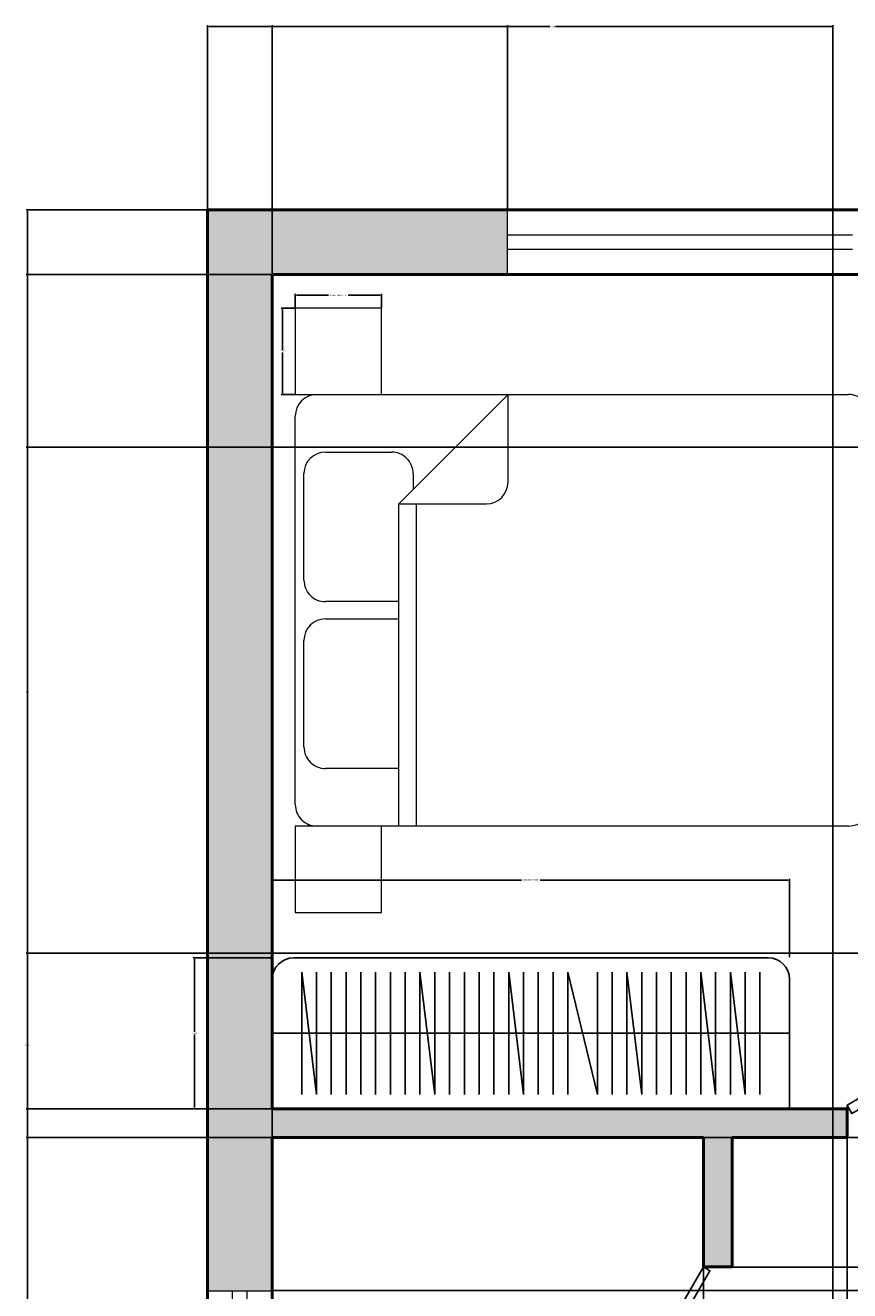
# Model space of a CAD drawing. Units: inches. Extents: x 3439 to 3988, y 1915 to 2284.
# Tile 2 of 7: x 3439 to 3554, y 2108 to 2284. Entities that reach past the tile are written whole.
import ezdxf

# ---------------------------------------------------------------- set-up
doc = ezdxf.new("R2010")
doc.units = ezdxf.units.IN
for name, color, linetype, lineweight in [('A-ANNO-DIMS', 2, 'Continuous', 18), ('A-DOOR', 3, 'Continuous', 25), ('A-FLOR-CASE', 8, 'Continuous', 25), ('A-FURN', 9, 'Continuous', 18), ('A-GLAZ', 4, 'Continuous', 18), ('A-WALL', 7, 'Continuous', 50)]:
    doc.layers.add(name, color=color, linetype=linetype, lineweight=lineweight)
doc.layers.add('A-WALL-PATT', color=18, linetype='Continuous', lineweight=13, true_color=0x000000)
doc.styles.get("Standard").update_dxf_attribs({"font": 'arial.ttf'})
doc.dimstyles.get("Standard").update_dxf_attribs({"dimtxt": 0.18, "dimasz": 0.18, "dimexe": 0.18, "dimexo": 0.0625, "dimgap": 0.09, "dimtad": 0, "dimtih": 1, "dimtoh": 1, "dimdec": 4, "dimzin": 0, "dimdsep": 46, "dimtxsty": 'Standard', "dimcen": 0.09, "dimadec": 0, "dimazin": 0, "dimtfac": 1, "dimtdec": 4, "dimtofl": 0, "dimtmove": 0, "dimatfit": 3, "dimfxl": 1, "dimtolj": 1, "dimtzin": 0, "dimarcsym": 0})

# ---------------------------------------------------------------- blocks, each defined once
blk = doc.blocks.new('*U4')
for p, q in [((0, 0), (0, -6)), ((40, 0), (40, -6))]:
    blk.add_line(p, q)
blk.add_lwpolyline([(0, 0), (34.64, 20), (35.52, 18.48), (0.87, -1.52)], close=True)
blk.add_arc((0, 0), 40, 0, 30)
blk = doc.blocks.new('*U5')
for p, q in [((0, 0), (0, 6)), ((40, 0), (40, 6))]:
    blk.add_line(p, q)
blk.add_lwpolyline([(0, 0), (34.64, -20), (35.52, -18.48), (0.87, 1.52)], close=True)
blk.add_arc((0, 0), 40, 330, 0)
blk = doc.blocks.new('Bed - Queen')
for p, q in [((3, 0), (56.99999, 0)), ((10.99999, -1.2), (25.79998, -1.2)), ((34.19999, -1.2), (48.99999, -1.2)), ((0, -77.00003), (0, -3)), ((59.99999, -3), (59.99999, -77.00003)), ((7.99999, -14.4), (7.99999, -4.2)), ((28.79998, -4.2), (28.79998, -14.4)), ((31.19999, -14.4), (31.19999, -4.2)), ((51.99999, -4.2), (51.99999, -13.4)), ((0, -14.4), (44.8, -14.4)), ((59.99999, -29.6), (44.8, -14.4)), ((44.8, -14.4), (44.8, -26.6)), ((44.8, -16.8), (0, -16.8)), ((48.99999, -16.4), (46.79936, -16.4)), ((47.8, -29.6), (59.99999, -29.6)), ((56.99999, -80.00003), (3, -80.00003))]:
    blk.add_line(p, q)
for centre, start, end in [((3, -3), 90, 180), ((56.99999, -3), 0, 90), ((10.99999, -4.2), 90, 180), ((25.79998, -4.2), 0, 90), ((34.19999, -4.2), 90, 180), ((48.99999, -4.2), 0, 90), ((48.99999, -13.4), 270, 0), ((47.8, -26.6), 180, 270), ((3, -77.00003), 180, 270), ((56.99999, -77.00003), 270, 0)]:
    blk.add_arc(centre, 3, start, end)
blk = doc.blocks.new('WINDOW-GLASS-48IN')
for p, q in [((0, 2), (48, 2)), ((0, 0), (48, 0))]:
    blk.add_line(p, q)
blk = doc.blocks.new('WINDOW-GLASS-24IN')
for p, q in [((0, 2), (24, 2)), ((0, 0), (24, 0))]:
    blk.add_line(p, q)
blk = doc.blocks.new('WARDROBE-72IN')
for p, q in [((3, 21), (69, 21)), ((0, 0), (0, 18)), ((4.11, 2), (4.11, 19)), ((4.11, 19), (6.17, 2)), ((6.17, 2), (6.17, 19)), ((8.23, 2), (8.23, 19)), ((10.28, 2), (10.28, 19)), ((12.34, 2), (12.34, 19)), ((14.4, 2), (14.4, 19)), ((16.45, 2), (16.45, 19)), ((18.51, 2), (18.51, 19)), ((20.57, 2), (20.57, 19)), ((20.57, 19), (22.62, 2)), ((22.62, 2), (22.62, 19)), ((24.68, 2), (24.68, 19)), ((26.74, 2), (26.74, 19)), ((28.79, 2), (28.79, 19)), ((30.85, 2), (30.85, 19)), ((32.91, 2), (32.91, 19)), ((32.91, 19), (34.97, 2)), ((34.97, 2), (34.97, 19)), ((37.02, 2), (37.02, 19)), ((39.08, 2), (39.08, 19)), ((41.14, 2), (41.14, 19)), ((41.14, 19), (45.25, 2)), ((45.25, 2), (45.25, 19)), ((47.31, 2), (47.31, 19)), ((49.36, 2), (49.36, 19)), ((49.36, 19), (51.42, 2)), ((51.42, 2), (51.42, 19)), ((53.48, 2), (53.48, 19)), ((55.53, 2), (55.53, 19)), ((57.59, 2), (57.59, 19)), ((59.65, 2), (59.65, 19)), ((59.65, 19), (61.7, 2)), ((61.7, 2), (61.7, 19)), ((63.76, 2), (63.76, 19)), ((63.76, 19), (65.82, 2)), ((65.82, 2), (65.82, 19)), ((67.87, 2), (67.87, 19)), ((72, 18), (72, 0)), ((0, 10.5), (72, 10.5)), ((72, 0), (0, 0))]:
    blk.add_line(p, q)
for centre, start, end in [((3, 18), 90, 180), ((69, 18), 0, 90)]:
    blk.add_arc(centre, 3, start, end)
blk = doc.blocks.new('NIGHTSTAND-12IN-SQUARE')
blk.add_lwpolyline([(0, 0), (12, 0), (12, 12), (0, 12)], close=True)
blk = doc.blocks.new('*D25')
at = {"layer": 'A-ANNO-DIMS', "color": 0, "lineweight": -2, "transparency": 16777216}
for p, q in [((3473.58, 2154.42), (3473.58, 2165.34)), ((3473.76, 2165.16), (3508.27, 2165.16)), ((3545.4, 2165.16), (3510.89, 2165.16)), ((3545.58, 2154.42), (3545.58, 2165.34))]:
    blk.add_line(p, q, dxfattribs=at)
at = {"layer": 'A-ANNO-DIMS', "color": 0, "transparency": 16777216}
for points in [[(3473.76, 2165.19), (3473.76, 2165.13), (3473.58, 2165.16)], [(3545.4, 2165.19), (3545.4, 2165.13), (3545.58, 2165.16)]]:
    blk.add_solid(points, dxfattribs=at)
at = {"layer": 'Defpoints', "color": 0, "transparency": 16777216}
for p in [(3545.58, 2165.16), (3473.58, 2154.36), (3545.58, 2154.36)]:
    blk.add_point(p, dxfattribs=at)
at = {"layer": 'A-ANNO-DIMS', "color": 0, "transparency": 16777216, "insert": (3509.58, 2165.16), "char_height": 0.18, "attachment_point": 5}
blk.add_mtext('\\A1;WARDROBE 72 TYP.', dxfattribs=at)
blk = doc.blocks.new('*D26')
at = {"layer": 'A-ANNO-DIMS', "color": 0, "lineweight": -2, "transparency": 16777216}
for p, q in [((3473.52, 2154.36), (3462.6, 2154.36)), ((3462.78, 2154.18), (3462.78, 2144.04)), ((3462.78, 2133.54), (3462.78, 2143.68)), ((3473.52, 2133.36), (3462.6, 2133.36))]:
    blk.add_line(p, q, dxfattribs=at)
at = {"layer": 'A-ANNO-DIMS', "color": 0, "transparency": 16777216}
for points in [[(3462.75, 2154.18), (3462.81, 2154.18), (3462.78, 2154.36)], [(3462.75, 2133.54), (3462.81, 2133.54), (3462.78, 2133.36)]]:
    blk.add_solid(points, dxfattribs=at)
at = {"layer": 'Defpoints', "color": 0, "transparency": 16777216}
for p in [(3462.78, 2154.36), (3473.58, 2154.36), (3473.58, 2133.36)]:
    blk.add_point(p, dxfattribs=at)
at = {"layer": 'A-ANNO-DIMS', "color": 0, "transparency": 16777216, "insert": (3462.78, 2143.86), "char_height": 0.18, "attachment_point": 5}
blk.add_mtext('\\A1;21 TYP.', dxfattribs=at)
blk = doc.blocks.new('*D29')
at = {"layer": 'A-ANNO-DIMS', "color": 0, "lineweight": -2, "transparency": 16777216}
for p, q in [((3476.8, 2244.73), (3476.8, 2246.65)), ((3476.98, 2246.47), (3481.42, 2246.47)), ((3488.62, 2246.47), (3484.17, 2246.47)), ((3488.8, 2244.73), (3488.8, 2246.65))]:
    blk.add_line(p, q, dxfattribs=at)
at = {"layer": 'A-ANNO-DIMS', "color": 0, "transparency": 16777216}
for points in [[(3476.98, 2246.5), (3476.98, 2246.44), (3476.8, 2246.47)], [(3488.62, 2246.5), (3488.62, 2246.44), (3488.8, 2246.47)]]:
    blk.add_solid(points, dxfattribs=at)
at = {"layer": 'Defpoints', "color": 0, "transparency": 16777216}
for p in [(3488.8, 2246.47), (3476.8, 2244.67), (3488.8, 2244.67)]:
    blk.add_point(p, dxfattribs=at)
at = {"layer": 'A-ANNO-DIMS', "color": 0, "transparency": 16777216, "insert": (3482.8, 2246.47), "char_height": 0.18, "attachment_point": 5}
blk.add_mtext('\\A1;NIGHTSTAND 12 TYP.', dxfattribs=at)
blk = doc.blocks.new('*D30')
at = {"layer": 'A-ANNO-DIMS', "color": 0, "lineweight": -2, "transparency": 16777216}
for p, q in [((3476.74, 2244.67), (3474.82, 2244.67)), ((3475, 2244.49), (3475, 2238.85)), ((3475, 2232.85), (3475, 2238.49)), ((3476.74, 2232.67), (3474.82, 2232.67))]:
    blk.add_line(p, q, dxfattribs=at)
at = {"layer": 'A-ANNO-DIMS', "color": 0, "transparency": 16777216}
for points in [[(3474.97, 2244.49), (3475.03, 2244.49), (3475, 2244.67)], [(3474.97, 2232.85), (3475.03, 2232.85), (3475, 2232.67)]]:
    blk.add_solid(points, dxfattribs=at)
at = {"layer": 'Defpoints', "color": 0, "transparency": 16777216}
for p in [(3475, 2244.67), (3476.8, 2244.67), (3476.8, 2232.67)]:
    blk.add_point(p, dxfattribs=at)
at = {"layer": 'A-ANNO-DIMS', "color": 0, "transparency": 16777216, "insert": (3475, 2238.67), "char_height": 0.18, "attachment_point": 5}
blk.add_mtext('\\A1;12 TYP.', dxfattribs=at)
blk = doc.blocks.new('*D46')
at = {"layer": 'A-ANNO-DIMS', "color": 0, "lineweight": -2, "transparency": 16777216}
for p, q in [((3464.52, 2258.36), (3439.35, 2258.36)), ((3439.53, 2258.18), (3439.53, 2099.54)), ((3439.53, 1940.54), (3439.53, 2099.18)), ((3464.52, 1940.36), (3439.35, 1940.36))]:
    blk.add_line(p, q, dxfattribs=at)
at = {"layer": 'A-ANNO-DIMS', "color": 0, "transparency": 16777216}
for points in [[(3439.5, 2258.18), (3439.56, 2258.18), (3439.53, 2258.36)], [(3439.5, 1940.54), (3439.56, 1940.54), (3439.53, 1940.36)]]:
    blk.add_solid(points, dxfattribs=at)
at = {"layer": 'Defpoints', "color": 0, "transparency": 16777216}
for p in [(3439.53, 2258.36), (3464.58, 2258.36), (3464.58, 1940.36)]:
    blk.add_point(p, dxfattribs=at)
at = {"layer": 'A-ANNO-DIMS', "color": 0, "transparency": 16777216, "insert": (3439.53, 2099.36), "char_height": 0.18, "attachment_point": 5}
blk.add_mtext('\\A1;318', dxfattribs=at)
blk = doc.blocks.new('*D47')
at = {"layer": 'A-ANNO-DIMS', "color": 0, "lineweight": -2, "transparency": 16777216}
for p, q in [((3473.58, 2249.3), (3473.58, 1915.13)), ((3589.58, 2249.3), (3589.58, 1915.13)), ((3473.76, 1915.31), (3531.3, 1915.31)), ((3589.4, 1915.31), (3531.86, 1915.31))]:
    blk.add_line(p, q, dxfattribs=at)
at = {"layer": 'A-ANNO-DIMS', "color": 0, "transparency": 16777216}
for points in [[(3473.76, 1915.34), (3473.76, 1915.28), (3473.58, 1915.31)], [(3589.4, 1915.34), (3589.4, 1915.28), (3589.58, 1915.31)]]:
    blk.add_solid(points, dxfattribs=at)
at = {"layer": 'Defpoints', "color": 0, "transparency": 16777216}
for p in [(3473.58, 2249.36), (3589.58, 2249.36), (3589.58, 1915.31)]:
    blk.add_point(p, dxfattribs=at)
at = {"layer": 'A-ANNO-DIMS', "color": 0, "transparency": 16777216, "insert": (3531.58, 1915.31), "char_height": 0.18, "attachment_point": 5}
blk.add_mtext('\\A1;116', dxfattribs=at)
blk = doc.blocks.new('*D55')
at = {"layer": 'A-ANNO-DIMS', "color": 0, "lineweight": -2, "transparency": 16777216}
for p, q in [((3473.52, 2249.36), (3439.35, 2249.36)), ((3439.53, 2249.18), (3439.53, 2191.54)), ((3439.53, 2133.54), (3439.53, 2191.18)), ((3473.52, 2133.36), (3439.35, 2133.36))]:
    blk.add_line(p, q, dxfattribs=at)
at = {"layer": 'A-ANNO-DIMS', "color": 0, "transparency": 16777216}
for points in [[(3439.5, 2249.18), (3439.56, 2249.18), (3439.53, 2249.36)], [(3439.5, 2133.54), (3439.56, 2133.54), (3439.53, 2133.36)]]:
    blk.add_solid(points, dxfattribs=at)
at = {"layer": 'Defpoints', "color": 0, "transparency": 16777216}
for p in [(3439.53, 2249.36), (3473.58, 2249.36), (3473.58, 2133.36)]:
    blk.add_point(p, dxfattribs=at)
at = {"layer": 'A-ANNO-DIMS', "color": 0, "transparency": 16777216, "insert": (3439.53, 2191.36), "char_height": 0.18, "attachment_point": 5}
blk.add_mtext('\\A1;116', dxfattribs=at)
blk = doc.blocks.new('*D56')
at = {"layer": 'A-ANNO-DIMS', "color": 0, "lineweight": -2, "transparency": 16777216}
for p, q in [((3473.52, 2129.36), (3439.35, 2129.36)), ((3439.53, 2129.18), (3439.53, 2093.54)), ((3439.53, 2057.54), (3439.53, 2093.18)), ((3473.52, 2057.36), (3439.35, 2057.36))]:
    blk.add_line(p, q, dxfattribs=at)
at = {"layer": 'A-ANNO-DIMS', "color": 0, "transparency": 16777216}
for points in [[(3439.5, 2129.18), (3439.56, 2129.18), (3439.53, 2129.36)], [(3439.5, 2057.54), (3439.56, 2057.54), (3439.53, 2057.36)]]:
    blk.add_solid(points, dxfattribs=at)
at = {"layer": 'Defpoints', "color": 0, "transparency": 16777216}
for p in [(3439.53, 2129.36), (3473.58, 2129.36), (3473.58, 2057.36)]:
    blk.add_point(p, dxfattribs=at)
at = {"layer": 'A-ANNO-DIMS', "color": 0, "transparency": 16777216, "insert": (3439.53, 2093.36), "char_height": 0.18, "attachment_point": 5}
blk.add_mtext('\\A1;72', dxfattribs=at)
blk = doc.blocks.new('*D61')
at = {"layer": 'A-ANNO-DIMS', "color": 0, "lineweight": -2, "transparency": 16777216}
for p, q in [((3473.58, 2129.3), (3473.58, 1915.13)), ((3533.58, 2129.3), (3533.58, 1915.13)), ((3473.76, 1915.31), (3503.36, 1915.31)), ((3533.4, 1915.31), (3503.8, 1915.31))]:
    blk.add_line(p, q, dxfattribs=at)
at = {"layer": 'A-ANNO-DIMS', "color": 0, "transparency": 16777216}
for points in [[(3473.76, 1915.34), (3473.76, 1915.28), (3473.58, 1915.31)], [(3533.4, 1915.34), (3533.4, 1915.28), (3533.58, 1915.31)]]:
    blk.add_solid(points, dxfattribs=at)
at = {"layer": 'Defpoints', "color": 0, "transparency": 16777216}
for p in [(3473.58, 2129.36), (3533.58, 2129.36), (3533.58, 1915.31)]:
    blk.add_point(p, dxfattribs=at)
at = {"layer": 'A-ANNO-DIMS', "color": 0, "transparency": 16777216, "insert": (3503.58, 1915.31), "char_height": 0.18, "attachment_point": 5}
blk.add_mtext('\\A1;60', dxfattribs=at)
blk = doc.blocks.new('*D66')
at = {"layer": 'A-ANNO-DIMS', "color": 0, "lineweight": -2, "transparency": 16777216}
for p, q in [((3464.58, 2258.42), (3464.58, 2284)), ((3464.76, 2283.82), (3485.05, 2283.82)), ((3506.14, 2283.82), (3485.85, 2283.82)), ((3506.32, 2258.42), (3506.32, 2284))]:
    blk.add_line(p, q, dxfattribs=at)
at = {"layer": 'A-ANNO-DIMS', "color": 0, "transparency": 16777216}
for points in [[(3464.76, 2283.85), (3464.76, 2283.79), (3464.58, 2283.82)], [(3506.14, 2283.85), (3506.14, 2283.79), (3506.32, 2283.82)]]:
    blk.add_solid(points, dxfattribs=at)
at = {"layer": 'Defpoints', "color": 0, "transparency": 16777216}
for p in [(3506.32, 2283.82), (3464.58, 2258.36), (3506.32, 2258.36)]:
    blk.add_point(p, dxfattribs=at)
at = {"layer": 'A-ANNO-DIMS', "color": 0, "transparency": 16777216, "insert": (3485.45, 2283.82), "char_height": 0.18, "attachment_point": 5}
blk.add_mtext('\\A1;41.74', dxfattribs=at)
blk = doc.blocks.new('*D72')
at = {"layer": 'A-ANNO-DIMS', "color": 0, "lineweight": -2, "transparency": 16777216}
for p, q in [((3473.58, 1949.42), (3473.58, 2284)), ((3473.76, 2283.82), (3512.21, 2283.82)), ((3551.44, 2283.82), (3512.99, 2283.82)), ((3551.62, 1949.42), (3551.62, 2284))]:
    blk.add_line(p, q, dxfattribs=at)
at = {"layer": 'A-ANNO-DIMS', "color": 0, "transparency": 16777216}
for points in [[(3473.76, 2283.85), (3473.76, 2283.79), (3473.58, 2283.82)], [(3551.44, 2283.85), (3551.44, 2283.79), (3551.62, 2283.82)]]:
    blk.add_solid(points, dxfattribs=at)
at = {"layer": 'Defpoints', "color": 0, "transparency": 16777216}
for p in [(3551.62, 2283.82), (3473.58, 1949.36), (3551.62, 1949.36)]:
    blk.add_point(p, dxfattribs=at)
at = {"layer": 'A-ANNO-DIMS', "color": 0, "transparency": 16777216, "insert": (3512.6, 2283.82), "char_height": 0.18, "attachment_point": 5}
blk.add_mtext('\\A1;78.04', dxfattribs=at)
blk = doc.blocks.new('*D77')
at = {"layer": 'A-ANNO-DIMS', "color": 0, "lineweight": -2, "transparency": 16777216}
for p, q in [((3473.64, 2129.36), (3987.81, 2129.36)), ((3987.63, 2129.18), (3987.63, 2118.9)), ((3987.63, 2108.25), (3987.63, 2118.53)), ((3473.64, 2108.07), (3987.81, 2108.07))]:
    blk.add_line(p, q, dxfattribs=at)
at = {"layer": 'A-ANNO-DIMS', "color": 0, "transparency": 16777216}
for points in [[(3987.6, 2129.18), (3987.66, 2129.18), (3987.63, 2129.36)], [(3987.6, 2108.25), (3987.66, 2108.25), (3987.63, 2108.07)]]:
    blk.add_solid(points, dxfattribs=at)
at = {"layer": 'Defpoints', "color": 0, "transparency": 16777216}
for p in [(3473.58, 2129.36), (3987.63, 2129.36), (3473.58, 2108.07)]:
    blk.add_point(p, dxfattribs=at)
at = {"layer": 'A-ANNO-DIMS', "color": 0, "transparency": 16777216, "insert": (3987.63, 2118.71), "char_height": 0.18, "attachment_point": 5}
blk.add_mtext('\\A1;21.295', dxfattribs=at)
blk = doc.blocks.new('*D78')
at = {"layer": 'A-ANNO-DIMS', "color": 0, "lineweight": -2, "transparency": 16777216}
for p, q in [((3553.58, 2129.3), (3553.58, 1915.13)), ((3583.58, 2129.3), (3583.58, 1915.13)), ((3553.76, 1915.31), (3568.36, 1915.31)), ((3583.4, 1915.31), (3568.8, 1915.31))]:
    blk.add_line(p, q, dxfattribs=at)
at = {"layer": 'A-ANNO-DIMS', "color": 0, "transparency": 16777216}
for points in [[(3553.76, 1915.34), (3553.76, 1915.28), (3553.58, 1915.31)], [(3583.4, 1915.34), (3583.4, 1915.28), (3583.58, 1915.31)]]:
    blk.add_solid(points, dxfattribs=at)
at = {"layer": 'Defpoints', "color": 0, "transparency": 16777216}
for p in [(3553.58, 2129.36), (3583.58, 2129.36), (3583.58, 1915.31)]:
    blk.add_point(p, dxfattribs=at)
at = {"layer": 'A-ANNO-DIMS', "color": 0, "transparency": 16777216, "insert": (3568.58, 1915.31), "char_height": 0.18, "attachment_point": 5}
blk.add_mtext('\\A1;30', dxfattribs=at)
blk = doc.blocks.new('*D82')
at = {"layer": 'A-ANNO-DIMS', "color": 0, "lineweight": -2, "transparency": 16777216}
for p, q in [((3537.64, 2129.36), (3987.81, 2129.36)), ((3987.63, 2129.18), (3987.63, 2120.54)), ((3987.63, 2111.54), (3987.63, 2120.18)), ((3537.64, 2111.36), (3987.81, 2111.36))]:
    blk.add_line(p, q, dxfattribs=at)
at = {"layer": 'A-ANNO-DIMS', "color": 0, "transparency": 16777216}
for points in [[(3987.6, 2129.18), (3987.66, 2129.18), (3987.63, 2129.36)], [(3987.6, 2111.54), (3987.66, 2111.54), (3987.63, 2111.36)]]:
    blk.add_solid(points, dxfattribs=at)
at = {"layer": 'Defpoints', "color": 0, "transparency": 16777216}
for p in [(3537.58, 2129.36), (3987.63, 2129.36), (3537.58, 2111.36)]:
    blk.add_point(p, dxfattribs=at)
at = {"layer": 'A-ANNO-DIMS', "color": 0, "transparency": 16777216, "insert": (3987.63, 2120.36), "char_height": 0.18, "attachment_point": 5}
blk.add_mtext('\\A1;18', dxfattribs=at)
blk = doc.blocks.new('*D83')
at = {"layer": 'A-ANNO-DIMS', "color": 0, "lineweight": -2, "transparency": 16777216}
for p, q in [((3537.64, 2111.36), (3987.81, 2111.36)), ((3987.63, 2111.18), (3987.63, 2099.54)), ((3987.63, 2087.54), (3987.63, 2099.18)), ((3537.64, 2087.36), (3987.81, 2087.36))]:
    blk.add_line(p, q, dxfattribs=at)
at = {"layer": 'A-ANNO-DIMS', "color": 0, "transparency": 16777216}
for points in [[(3987.6, 2111.18), (3987.66, 2111.18), (3987.63, 2111.36)], [(3987.6, 2087.54), (3987.66, 2087.54), (3987.63, 2087.36)]]:
    blk.add_solid(points, dxfattribs=at)
at = {"layer": 'Defpoints', "color": 0, "transparency": 16777216}
for p in [(3537.58, 2111.36), (3987.63, 2111.36), (3537.58, 2087.36)]:
    blk.add_point(p, dxfattribs=at)
at = {"layer": 'A-ANNO-DIMS', "color": 0, "transparency": 16777216, "insert": (3987.63, 2099.36), "char_height": 0.18, "attachment_point": 5}
blk.add_mtext('\\A1;24', dxfattribs=at)
blk = doc.blocks.new('*D96')
at = {"layer": 'A-ANNO-DIMS', "color": 0, "lineweight": -2, "transparency": 16777216}
for p, q in [((3793.87, 2249.36), (3439.35, 2249.36)), ((3439.53, 2249.18), (3439.53, 2237.54)), ((3439.53, 2225.54), (3439.53, 2237.18)), ((3769.87, 2225.36), (3439.35, 2225.36))]:
    blk.add_line(p, q, dxfattribs=at)
at = {"layer": 'A-ANNO-DIMS', "color": 0, "transparency": 16777216}
for points in [[(3439.5, 2249.18), (3439.56, 2249.18), (3439.53, 2249.36)], [(3439.5, 2225.54), (3439.56, 2225.54), (3439.53, 2225.36)]]:
    blk.add_solid(points, dxfattribs=at)
at = {"layer": 'Defpoints', "color": 0, "transparency": 16777216}
for p in [(3439.53, 2249.36), (3793.93, 2249.36), (3769.93, 2225.36)]:
    blk.add_point(p, dxfattribs=at)
at = {"layer": 'A-ANNO-DIMS', "color": 0, "transparency": 16777216, "insert": (3439.53, 2237.36), "char_height": 0.18, "attachment_point": 5}
blk.add_mtext('\\A1;24', dxfattribs=at)
blk = doc.blocks.new('*D98')
at = {"layer": 'A-ANNO-DIMS', "color": 0, "lineweight": -2, "transparency": 16777216}
for p, q in [((3889.52, 2154.99), (3439.35, 2154.99)), ((3439.53, 2154.81), (3439.53, 2142.36)), ((3439.53, 2129.54), (3439.53, 2141.99)), ((3889.52, 2129.36), (3439.35, 2129.36))]:
    blk.add_line(p, q, dxfattribs=at)
at = {"layer": 'A-ANNO-DIMS', "color": 0, "transparency": 16777216}
for points in [[(3439.5, 2154.81), (3439.56, 2154.81), (3439.53, 2154.99)], [(3439.5, 2129.54), (3439.56, 2129.54), (3439.53, 2129.36)]]:
    blk.add_solid(points, dxfattribs=at)
at = {"layer": 'Defpoints', "color": 0, "transparency": 16777216}
for p in [(3889.58, 2154.99), (3439.53, 2129.36), (3889.58, 2129.36)]:
    blk.add_point(p, dxfattribs=at)
at = {"layer": 'A-ANNO-DIMS', "color": 0, "transparency": 16777216, "insert": (3439.53, 2142.18), "char_height": 0.18, "attachment_point": 5}
blk.add_mtext('\\A1;25.63', dxfattribs=at)

msp = doc.modelspace()

# ---------------------------------------------------------------- hatches: boundary and pattern name
at = {"layer": 'A-WALL-PATT'}
h = msp.add_hatch(color=256, dxfattribs=at)
h.dxf.hatch_style = 1
h.paths.add_polyline_path([(3506.3179, 2258.3617), (3464.5815, 2258.3617), (3464.5815, 2108.0664), (3473.5815, 2108.0664), (3473.5815, 2129.3617), (3533.5815, 2129.3617), (3533.5815, 2111.3617), (3537.1815, 2111.3617), (3537.5815, 2111.3617), (3537.5815, 2129.3617), (3553.5815, 2129.3617), (3553.5815, 2133.3617), (3473.5815, 2133.3617), (3473.5815, 2249.3617), (3506.3179, 2249.3617)])

# ---------------------------------------------------------------- linework, layer by layer
at = {"layer": 'A-GLAZ'}
for points in [[(3506.3179, 2249.3617), (3506.3179, 2258.3617)], [(3464.5815, 2108.0664), (3473.5815, 2108.0664)]]:
    msp.add_lwpolyline(points, dxfattribs=at)
at = {"layer": 'A-WALL'}
for p, q in [((3473.5815, 2249.3617), (3589.5815, 2249.3617)), ((3473.5815, 2133.3617), (3473.5815, 2249.3617)), ((3473.5815, 2133.3617), (3553.5815, 2133.3617)), ((3553.5815, 2133.3617), (3553.5815, 2129.3617)), ((3473.5815, 2129.3617), (3533.5815, 2129.3617)), ((3473.5815, 2057.3617), (3473.5815, 2129.3617)), ((3533.5815, 2111.3617), (3533.5815, 2129.3617)), ((3537.5815, 2129.3617), (3553.5815, 2129.3617)), ((3537.5815, 2111.3617), (3537.5815, 2129.3617)), ((3537.5815, 2111.3617), (3533.5815, 2111.3617))]:
    msp.add_line(p, q, dxfattribs=at)
msp.add_lwpolyline([(3719.5815, 1940.3617), (3464.5815, 1940.3617), (3464.5815, 2258.3617), (3803.9319, 2258.3617)], dxfattribs=at)

# ---------------------------------------------------------------- block references
at = {"layer": 'A-DOOR', "xscale": 0.75, "yscale": 0.75, "zscale": 0.75}
msp.add_blockref('*U4', (3553.5815, 2133.8617), dxfattribs=at)
at = {"layer": 'A-DOOR', "xscale": 0.6000000000000001, "yscale": 0.6000000000000001, "zscale": 0.6000000000000001, "rotation": 270}
msp.add_blockref('*U5', (3533.5815, 2111.3617), dxfattribs=at)
at = {"layer": 'A-FLOR-CASE'}
msp.add_blockref('WARDROBE-72IN', (3473.5815, 2133.3617), dxfattribs=at)
at = {"layer": 'A-FURN'}
for p in [(3476.798, 2232.669), (3476.798, 2160.669)]:
    msp.add_blockref('NIGHTSTAND-12IN-SQUARE', p, dxfattribs=at)
at = {"layer": 'A-FURN', "rotation": 89.99999999999999}
msp.add_blockref('Bed - Queen', (3476.798, 2172.669), dxfattribs=at)
at = {"layer": 'A-GLAZ'}
msp.add_blockref('WINDOW-GLASS-48IN', (3506.3179, 2252.8617), dxfattribs=at)
at = {"layer": 'A-GLAZ', "rotation": 90.0000000000043}
msp.add_blockref('WINDOW-GLASS-24IN', (3470.0815, 2084.0664), dxfattribs=at)

# ---------------------------------------------------------------- dimensions: what is measured, and where the dimension line sits
at = {"layer": 'A-ANNO-DIMS'}
for base, p1, p2, override, picture, middle in [((3506.3179, 2283.8228), (3464.5815, 2258.3617), (3506.3179, 2258.3617), {"dimdec": 2, "dimlfac": 1, "dimrnd": 0, "dimzin": 0, "dimdsep": 46, "dimlunit": 2}, '*D66', (3485.4497, 2283.8228)), ((3551.6168, 2283.8228), (3473.5815, 1949.3617), (3551.6168, 1949.3617), {"dimdec": 2, "dimlfac": 1, "dimrnd": 0, "dimzin": 0, "dimdsep": 46, "dimlunit": 2}, '*D72', (3512.5992, 2283.8228)), ((3589.5815, 1915.3117), (3473.5815, 2249.3617), (3589.5815, 2249.3617), {"dimdec": 0, "dimlfac": 1, "dimrnd": 0, "dimzin": 0, "dimdsep": 46, "dimlunit": 2}, '*D47', (3531.5815, 1915.3117)), ((3533.5815, 1915.3117), (3473.5815, 2129.3617), (3533.5815, 2129.3617), {"dimdec": 0, "dimlfac": 1, "dimrnd": 0, "dimzin": 0, "dimdsep": 46, "dimlunit": 2}, '*D61', (3503.5815, 1915.3117)), ((3583.5815, 1915.3117), (3553.5815, 2129.3617), (3583.5815, 2129.3617), {"dimdec": 0, "dimlfac": 1, "dimrnd": 0, "dimzin": 0, "dimdsep": 46, "dimlunit": 2}, '*D78', (3568.5815, 1915.3117))]:
    dim = msp.add_linear_dim(base=base, p1=p1, p2=p2, dimstyle='Standard', override=override, dxfattribs=at)
    dim.commit()
    dim.dimension.update_dxf_attribs({"geometry": picture, "text_midpoint": middle})
for base, p1, p2, override, picture, middle in [((3439.5315, 2258.3617), (3464.5815, 1940.3617), (3464.5815, 2258.3617), {"dimdec": 0, "dimlfac": 1, "dimrnd": 0, "dimzin": 0, "dimdsep": 46, "dimlunit": 2}, '*D46', (3439.5315, 2099.3617)), ((3439.5315, 2249.3617), (3473.5815, 2133.3617), (3473.5815, 2249.3617), {"dimdec": 0, "dimlfac": 1, "dimrnd": 0, "dimzin": 0, "dimdsep": 46, "dimlunit": 2}, '*D55', (3439.5315, 2191.3617)), ((3439.5315, 2249.3617), (3769.9319, 2225.3617), (3793.9319, 2249.3617), {"dimdec": 0, "dimlfac": 1, "dimrnd": 0, "dimzin": 0, "dimdsep": 46, "dimlunit": 2}, '*D96', (3439.5315, 2237.3617)), ((3439.5315, 2129.3617), (3889.5815, 2154.9906), (3889.5815, 2129.3617), {"dimdec": 2, "dimlfac": 1, "dimrnd": 0, "dimzin": 0, "dimdsep": 46, "dimlunit": 2}, '*D98', (3439.5315, 2142.1761)), ((3439.5315, 2129.3617), (3473.5815, 2057.3617), (3473.5815, 2129.3617), {"dimdec": 0, "dimlfac": 1, "dimrnd": 0, "dimzin": 0, "dimdsep": 46, "dimlunit": 2}, '*D56', (3439.5315, 2093.3617)), ((3987.6315, 2129.3617), (3473.5815, 2108.0664), (3473.5815, 2129.3617), {"dimdec": 3, "dimlfac": 1, "dimrnd": 0, "dimzin": 0, "dimdsep": 46, "dimlunit": 2}, '*D77', (3987.6315, 2118.7141)), ((3987.6315, 2129.3617), (3537.5815, 2111.3617), (3537.5815, 2129.3617), {"dimdec": 0, "dimlfac": 1, "dimrnd": 0, "dimzin": 0, "dimdsep": 46, "dimlunit": 2}, '*D82', (3987.6315, 2120.3617)), ((3987.6315, 2111.3617), (3537.5815, 2087.3617), (3537.5815, 2111.3617), {"dimdec": 0, "dimlfac": 1, "dimrnd": 0, "dimzin": 0, "dimdsep": 46, "dimlunit": 2}, '*D83', (3987.6315, 2099.3617))]:
    dim = msp.add_linear_dim(base=base, p1=p1, p2=p2, angle=90, dimstyle='Standard', override=override, dxfattribs=at)
    dim.commit()
    dim.dimension.update_dxf_attribs({"geometry": picture, "text_midpoint": middle})
for base, p1, p2, text, picture, middle in [((3488.798, 2246.469), (3476.798, 2244.669), (3488.798, 2244.669), 'NIGHTSTAND <> TYP.', '*D29', (3482.798, 2246.469)), ((3545.5815, 2165.1617), (3473.5815, 2154.3617), (3545.5815, 2154.3617), 'WARDROBE <> TYP.', '*D25', (3509.5815, 2165.1617))]:
    dim = msp.add_linear_dim(base=base, p1=p1, p2=p2, text=text, dimstyle='Standard', override={"dimdec": 0, "dimlfac": 1, "dimrnd": 0, "dimzin": 0, "dimdsep": 46, "dimlunit": 2}, dxfattribs=at)
    dim.commit()
    dim.dimension.update_dxf_attribs({"geometry": picture, "text_midpoint": middle})
for base, p1, p2, picture, middle in [((3474.998, 2244.669), (3476.798, 2232.669), (3476.798, 2244.669), '*D30', (3474.998, 2238.669)), ((3462.7815, 2154.3617), (3473.5815, 2133.3617), (3473.5815, 2154.3617), '*D26', (3462.7815, 2143.8617))]:
    dim = msp.add_linear_dim(base=base, p1=p1, p2=p2, angle=90, text='<> TYP.', dimstyle='Standard', override={"dimdec": 0, "dimlfac": 1, "dimrnd": 0, "dimzin": 0, "dimdsep": 46, "dimlunit": 2}, dxfattribs=at)
    dim.commit()
    dim.dimension.update_dxf_attribs({"geometry": picture, "text_midpoint": middle})

doc.saveas('drawing.dxf')
